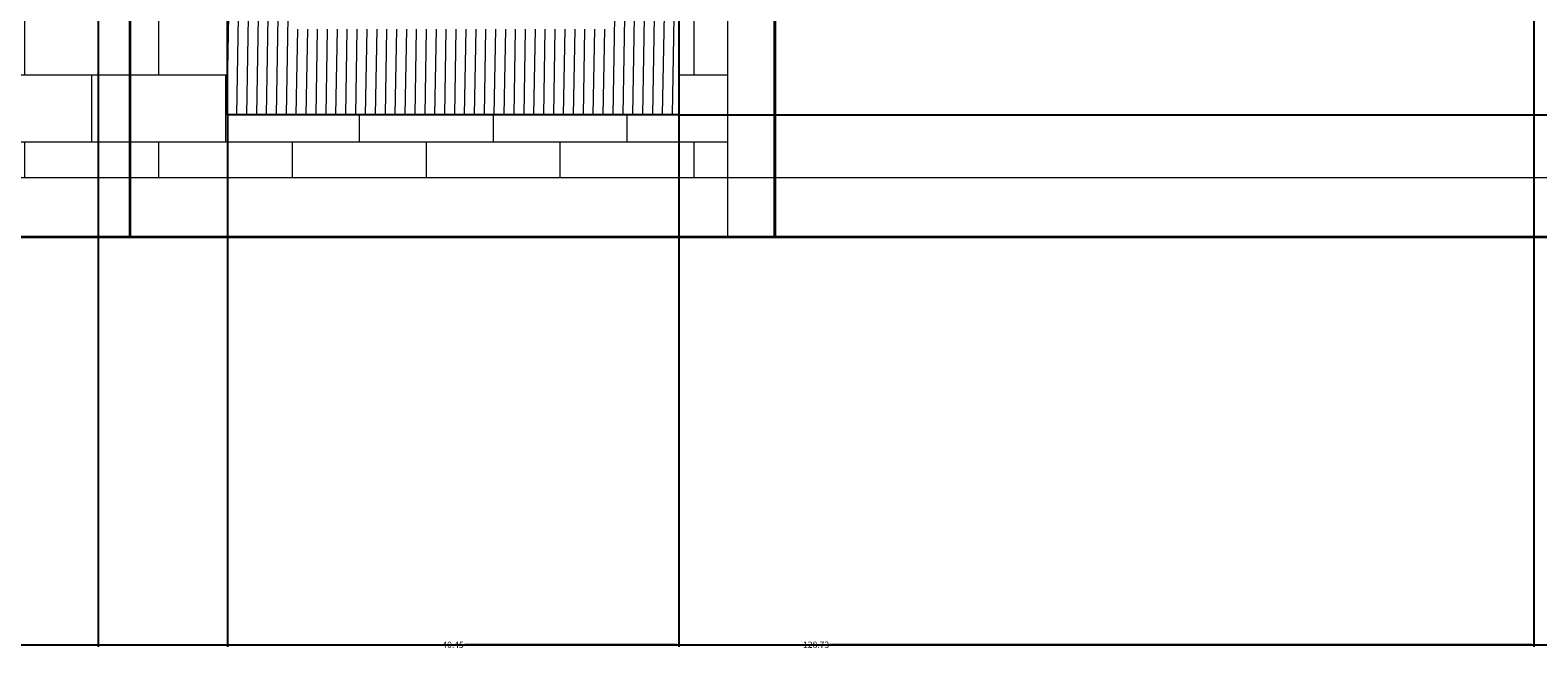
# Model space of a CAD drawing. Units: inches. Extents: x -26 to 776, y -22 to 650.
# Tile 14 of 62: x 222 to 358, y -22 to 34. Entities that reach past the tile are written whole.
import ezdxf

# ---------------------------------------------------------------- set-up
doc = ezdxf.new("R2010")
doc.units = ezdxf.units.IN
doc.header["$MEASUREMENT"] = 0
for name, color, linetype, lineweight in [('A-ANNO-DIMS', 2, 'Continuous', 18), ('A-DETL-PATT', 8, 'Continuous', 13), ('A-DOOR', 3, 'Continuous', 25), ('A-WALL', 7, 'Continuous', 35), ('A-WALL-PATT', 8, 'Continuous', 13), ('A-WALL-TRIM', 7, 'Continuous', 18), ('C-TOPO', 7, 'Continuous', 35)]:
    doc.layers.add(name, color=color, linetype=linetype, lineweight=lineweight)
doc.styles.get("Standard").update_dxf_attribs({"font": 'arial.ttf'})
doc.dimstyles.get("Standard").update_dxf_attribs({"dimtxt": 0.5625, "dimasz": 0.18, "dimexe": 0.18, "dimexo": 0.0625, "dimgap": 0.09, "dimtad": 0, "dimtih": 1, "dimtoh": 1, "dimdec": 4, "dimzin": 0, "dimdsep": 46, "dimlunit": 4, "dimtxsty": 'Standard', "dimcen": 0.09, "dimadec": 0, "dimazin": 0, "dimtfac": 1, "dimtdec": 4, "dimtofl": 0, "dimtmove": 0, "dimatfit": 3, "dimfxl": 1, "dimtolj": 1, "dimtzin": 0, "dimarcsym": 0})

# ---------------------------------------------------------------- blocks, each defined once
blk = doc.blocks.new('*D13')
at = {"layer": 'A-ANNO-DIMS', "color": 0, "lineweight": -2, "transparency": 16777216}
for p, q in [((738.75, 50.79), (738.75, -21.31)), ((11.11, 15.42), (11.11, -21.31)), ((11.29, -21.13), (373.89, -21.13)), ((738.57, -21.13), (375.97, -21.13))]:
    blk.add_line(p, q, dxfattribs=at)
at = {"layer": 'A-ANNO-DIMS', "color": 0, "transparency": 16777216}
for points in [[(11.29, -21.1), (11.29, -21.16), (11.11, -21.13)], [(738.57, -21.1), (738.57, -21.16), (738.75, -21.13)]]:
    blk.add_solid(points, dxfattribs=at)
at = {"layer": 'Defpoints', "color": 0, "transparency": 16777216}
for p in [(738.75, 50.85), (11.11, 15.48), (738.75, -21.13)]:
    blk.add_point(p, dxfattribs=at)
at = {"layer": 'A-ANNO-DIMS', "color": 0, "transparency": 16777216, "insert": (374.93, -21.13), "char_height": 0.562, "attachment_point": 5}
blk.add_mtext('\\A1;727.6', dxfattribs=at)
blk = doc.blocks.new('*D29')
at = {"layer": 'A-ANNO-DIMS', "color": 0, "lineweight": -2, "transparency": 16777216}
for p, q in [((240.17, 26.36), (240.17, -21.31)), ((280.62, 26.36), (280.62, -21.31)), ((240.35, -21.13), (259.34, -21.13)), ((280.44, -21.13), (261.44, -21.13))]:
    blk.add_line(p, q, dxfattribs=at)
at = {"layer": 'A-ANNO-DIMS', "color": 0, "transparency": 16777216}
for points in [[(240.35, -21.1), (240.35, -21.16), (240.17, -21.13)], [(280.44, -21.1), (280.44, -21.16), (280.62, -21.13)]]:
    blk.add_solid(points, dxfattribs=at)
at = {"layer": 'Defpoints', "color": 0, "transparency": 16777216}
for p in [(240.17, 26.42), (280.62, 26.42), (280.62, -21.13)]:
    blk.add_point(p, dxfattribs=at)
at = {"layer": 'A-ANNO-DIMS', "color": 0, "transparency": 16777216, "insert": (260.39, -21.13), "char_height": 0.562, "attachment_point": 5}
blk.add_mtext('\\A1;40.45', dxfattribs=at)
blk = doc.blocks.new('*D30')
at = {"layer": 'A-ANNO-DIMS', "color": 0, "lineweight": -2, "transparency": 16777216}
for p, q in [((280.68, 144.84), (775.34, 144.84)), ((775.16, 144.66), (775.16, 86.01)), ((775.16, 26.6), (775.16, 85.25)), ((280.68, 26.42), (775.34, 26.42))]:
    blk.add_line(p, q, dxfattribs=at)
at = {"layer": 'A-ANNO-DIMS', "color": 0, "transparency": 16777216}
for points in [[(775.13, 144.66), (775.19, 144.66), (775.16, 144.84)], [(775.13, 26.6), (775.19, 26.6), (775.16, 26.42)]]:
    blk.add_solid(points, dxfattribs=at)
at = {"layer": 'Defpoints', "color": 0, "transparency": 16777216}
for p in [(280.62, 144.84), (775.16, 144.84), (280.62, 26.42)]:
    blk.add_point(p, dxfattribs=at)
at = {"layer": 'A-ANNO-DIMS', "color": 0, "transparency": 16777216, "insert": (775.16, 85.63), "char_height": 0.562, "attachment_point": 5}
blk.add_mtext('\\A1;118.41', dxfattribs=at)
blk = doc.blocks.new('*D34')
at = {"layer": 'A-ANNO-DIMS', "color": 0, "lineweight": -2, "transparency": 16777216}
for p, q in [((228.57, 528.3), (228.57, -21.31)), ((357.3, 528.36), (357.3, -21.31)), ((228.75, -21.13), (291.71, -21.13)), ((357.12, -21.13), (294.17, -21.13))]:
    blk.add_line(p, q, dxfattribs=at)
at = {"layer": 'A-ANNO-DIMS', "color": 0, "transparency": 16777216}
for points in [[(228.75, -21.1), (228.75, -21.16), (228.57, -21.13)], [(357.12, -21.1), (357.12, -21.16), (357.3, -21.13)]]:
    blk.add_solid(points, dxfattribs=at)
at = {"layer": 'Defpoints', "color": 0, "transparency": 16777216}
for p in [(228.57, 528.36), (357.3, 528.42), (357.3, -21.13)]:
    blk.add_point(p, dxfattribs=at)
at = {"layer": 'A-ANNO-DIMS', "color": 0, "transparency": 16777216, "insert": (292.94, -21.13), "char_height": 0.562, "attachment_point": 5}
blk.add_mtext('\\A1;128.73', dxfattribs=at)
blk = doc.blocks.new('*D37')
at = {"layer": 'A-ANNO-DIMS', "color": 0, "lineweight": -2, "transparency": 16777216}
for p, q in [((231.36, 159.48), (-25.48, 159.48)), ((-25.3, 159.3), (-25.3, 87.85)), ((-25.3, 15.66), (-25.3, 87.11)), ((217.89, 15.48), (-25.48, 15.48))]:
    blk.add_line(p, q, dxfattribs=at)
at = {"layer": 'A-ANNO-DIMS', "color": 0, "transparency": 16777216}
for points in [[(-25.33, 159.3), (-25.27, 159.3), (-25.3, 159.48)], [(-25.33, 15.66), (-25.27, 15.66), (-25.3, 15.48)]]:
    blk.add_solid(points, dxfattribs=at)
at = {"layer": 'Defpoints', "color": 0, "transparency": 16777216}
for p in [(-25.3, 159.48), (231.42, 159.48), (217.95, 15.48)]:
    blk.add_point(p, dxfattribs=at)
at = {"layer": 'A-ANNO-DIMS', "color": 0, "transparency": 16777216, "insert": (-25.3, 87.48), "char_height": 0.562, "attachment_point": 5}
blk.add_mtext('\\A1;144', dxfattribs=at)
blk = doc.blocks.new('*D38')
at = {"layer": 'A-ANNO-DIMS', "color": 0, "lineweight": -2, "transparency": 16777216}
for p, q in [((280.68, 26.42), (775.34, 26.42)), ((775.16, 26.24), (775.16, 21.33)), ((775.16, 15.66), (775.16, 20.58)), ((289.3, 15.48), (775.34, 15.48))]:
    blk.add_line(p, q, dxfattribs=at)
at = {"layer": 'A-ANNO-DIMS', "color": 0, "transparency": 16777216}
for points in [[(775.13, 26.24), (775.19, 26.24), (775.16, 26.42)], [(775.13, 15.66), (775.19, 15.66), (775.16, 15.48)]]:
    blk.add_solid(points, dxfattribs=at)
at = {"layer": 'Defpoints', "color": 0, "transparency": 16777216}
for p in [(280.62, 26.42), (775.16, 26.42), (289.24, 15.48)]:
    blk.add_point(p, dxfattribs=at)
at = {"layer": 'A-ANNO-DIMS', "color": 0, "transparency": 16777216, "insert": (775.16, 20.95), "char_height": 0.562, "attachment_point": 5}
blk.add_mtext('\\A1;10.942', dxfattribs=at)
blk = doc.blocks.new('*D39')
at = {"layer": 'A-ANNO-DIMS', "color": 0, "lineweight": -2, "transparency": 16777216}
for p, q in [((289.24, 15.54), (289.24, 649.86)), ((289.42, 649.68), (356.48, 649.68)), ((425.56, 649.68), (358.51, 649.68)), ((425.74, 15.54), (425.74, 649.86))]:
    blk.add_line(p, q, dxfattribs=at)
at = {"layer": 'A-ANNO-DIMS', "color": 0, "transparency": 16777216}
for points in [[(289.42, 649.71), (289.42, 649.65), (289.24, 649.68)], [(425.56, 649.71), (425.56, 649.65), (425.74, 649.68)]]:
    blk.add_solid(points, dxfattribs=at)
at = {"layer": 'Defpoints', "color": 0, "transparency": 16777216}
for p in [(425.74, 649.68), (289.24, 15.48), (425.74, 15.48)]:
    blk.add_point(p, dxfattribs=at)
at = {"layer": 'A-ANNO-DIMS', "color": 0, "transparency": 16777216, "insert": (357.49, 649.68), "char_height": 0.562, "attachment_point": 5}
blk.add_mtext('\\A1;136.5', dxfattribs=at)
blk = doc.blocks.new('*D44')
at = {"layer": 'A-ANNO-DIMS', "color": 0, "lineweight": -2, "transparency": 16777216}
for p, q in [((231.42, 15.54), (231.42, 649.86)), ((231.6, 649.68), (234.98, 649.68)), ((239.99, 649.68), (236.61, 649.68)), ((240.17, 26.49), (240.17, 649.86))]:
    blk.add_line(p, q, dxfattribs=at)
at = {"layer": 'A-ANNO-DIMS', "color": 0, "transparency": 16777216}
for points in [[(231.6, 649.71), (231.6, 649.65), (231.42, 649.68)], [(239.99, 649.71), (239.99, 649.65), (240.17, 649.68)]]:
    blk.add_solid(points, dxfattribs=at)
at = {"layer": 'Defpoints', "color": 0, "transparency": 16777216}
for p in [(240.17, 649.68), (240.17, 26.42), (231.42, 15.48)]:
    blk.add_point(p, dxfattribs=at)
at = {"layer": 'A-ANNO-DIMS', "color": 0, "transparency": 16777216, "insert": (235.8, 649.68), "char_height": 0.562, "attachment_point": 5}
blk.add_mtext('\\A1;8.74', dxfattribs=at)

msp = doc.modelspace()

# ---------------------------------------------------------------- hatches: boundary and pattern name
at = {"layer": 'A-DETL-PATT'}
h = msp.add_hatch(dxfattribs=at)
h.set_pattern_fill('ANSI31', color=256, scale=7.1, angle=44)
h.paths.add_polyline_path([(231.4249, 197.3298), (216.1056, 197.3298), (216.1056, 159.4824), (231.4249, 159.4824)])
h.paths.add_polyline_path([(236.4647, 197.3298), (231.4249, 197.3298), (231.4249, 159.4824), (276.1134, 159.4824), (276.1134, 171.4173), (236.4647, 171.4173)])
h.paths.add_polyline_path([(259.7413, 197.3298), (236.4647, 197.3298), (236.4647, 171.4173), (259.7413, 171.4173)], flags=17)
h.paths.add_polyline_path([(276.1134, 197.3298), (261.7413, 197.3298), (261.7413, 171.4173), (276.1134, 171.4173)], flags=17)
h.paths.add_polyline_path([(217.9529, 147.0781), (22.8891, 147.0781), (22.8891, 138.3844), (217.9529, 138.3844)])
h.paths.add_polyline_path([(285.0179, 152.3087), (285.0179, 159.4824), (231.4249, 159.4824), (240.1654, 144.8359), (280.6173, 144.8359)])
h.paths.add_polyline_path([(280.6173, 144.8359), (240.1654, 144.8359), (240.1654, 26.4239), (280.6173, 26.4239)])
h.paths.add_polyline_path([(274.6644, 134.8811), (274.6644, 34.0885), (245.7207, 34.0885), (245.7207, 134.8811)], flags=16)
h.paths.add_polyline_path([(285.0179, 303.3046), (236.4647, 303.3046), (236.4647, 294.4171), (285.0179, 294.4171)])
h.paths.add_polyline_path([(285.0179, 446.0063), (236.4647, 446.0063), (236.4647, 437.1188), (285.0179, 437.1188)])
at = {"layer": 'A-WALL-PATT'}
h = msp.add_hatch(dxfattribs=at)
h.set_pattern_fill('AR-B816', color=256, scale=4.5)
h.paths.add_polyline_path([(425.7434, 448.2114), (289.2424, 496.9554), (289.2424, 458.1203), (289.2424, 291.1798), (289.2424, 20.7937), (425.7434, 20.7937), (425.7434, 283.2492)])
h = msp.add_hatch(dxfattribs=at)
h.set_pattern_fill('AR-B816', color=256, scale=0.75)
h.paths.add_polyline_path([(82.134, 209.6413), (11.1074, 209.6413), (11.1074, 159.4824), (82.134, 159.4824)])
h.paths.add_polyline_path([(231.4249, 209.6413), (209.091, 209.6413), (209.091, 159.4824), (214.1056, 159.4824), (214.1056, 199.3298), (231.4249, 199.3298)])
h.paths.add_polyline_path([(231.4249, 159.4824), (11.1074, 159.4824), (11.1074, 22.5014), (22.8891, 22.5014), (22.8891, 147.0781), (217.9529, 147.0781), (217.9529, 20.7937), (231.4249, 20.7937)])
h.paths.add_polyline_path([(285.0179, 152.3087), (280.6173, 144.8359), (280.6173, 26.4239), (240.1654, 26.4239), (240.1654, 144.8359), (231.4249, 159.4824), (231.4249, 20.7937), (285.0179, 20.7937)])

# ---------------------------------------------------------------- linework, layer by layer
at = {"layer": 'A-DOOR'}
msp.add_lwpolyline([(240.1654, 144.8359), (280.6173, 144.8359), (280.6173, 26.4239), (240.1654, 26.4239)], close=True, dxfattribs=at)
at = {"layer": 'A-WALL'}
for p, q in [((289.2424, 291.1798), (289.2424, 15.4824)), ((231.4249, 159.4824), (231.4249, 15.4824)), ((289.2424, 15.4824), (289.2424, 159.4824))]:
    msp.add_line(p, q, dxfattribs=at)
at = {"layer": 'A-WALL-TRIM'}
for p, q in [((285.0179, 15.4824), (285.0179, 249.6598)), ((217.9529, 20.7937), (425.7434, 20.7937))]:
    msp.add_line(p, q, dxfattribs=at)
at = {"layer": 'C-TOPO'}
for p, q in [((214.0443, 15.4824), (289.2424, 15.4824)), ((289.2424, 15.4824), (425.7434, 15.4824))]:
    msp.add_line(p, q, dxfattribs=at)

# ---------------------------------------------------------------- dimensions: what is measured, and where the dimension line sits
at = {"layer": 'A-ANNO-DIMS'}
for base, p1, p2, override, picture, middle in [((240.1654, 649.6763), (231.4249, 15.4824), (240.1654, 26.4239), {"dimdec": 2, "dimlfac": 1, "dimrnd": 0, "dimzin": 0, "dimdsep": 46, "dimlunit": 2}, '*D44', (235.7952, 649.6763)), ((425.7434, 649.6763), (289.2424, 15.4824), (425.7434, 15.4824), {"dimdec": 1, "dimlfac": 1, "dimrnd": 0, "dimzin": 0, "dimdsep": 46, "dimlunit": 2}, '*D39', (357.4929, 649.6763)), ((357.3034, -21.1349), (228.5733, 528.3585), (357.3034, 528.4233), {"dimdec": 2, "dimlfac": 1, "dimrnd": 0, "dimzin": 0, "dimdsep": 46, "dimlunit": 2}, '*D34', (292.9384, -21.1349)), ((738.7503, -21.1349), (11.1074, 15.4824), (738.7503, 50.8482), {"dimdec": 1, "dimlfac": 1, "dimrnd": 0, "dimzin": 0, "dimdsep": 46, "dimlunit": 2}, '*D13', (374.9289, -21.1349)), ((280.6173, -21.1349), (240.1654, 26.4239), (280.6173, 26.4239), {"dimdec": 2, "dimlfac": 1, "dimrnd": 0, "dimzin": 0, "dimdsep": 46, "dimlunit": 2}, '*D29', (260.3914, -21.1349))]:
    dim = msp.add_linear_dim(base=base, p1=p1, p2=p2, dimstyle='Standard', override=override, dxfattribs=at)
    dim.commit()
    dim.dimension.update_dxf_attribs({"geometry": picture, "text_midpoint": middle})
for base, p1, p2, override, picture, middle in [((-25.2976, 159.4824), (217.9529, 15.4824), (231.4249, 159.4824), {"dimdec": 0, "dimlfac": 1, "dimrnd": 0, "dimzin": 0, "dimdsep": 46, "dimlunit": 2}, '*D37', (-25.2976, 87.4824)), ((775.1553, 144.8359), (280.6173, 26.4239), (280.6173, 144.8359), {"dimdec": 2, "dimlfac": 1, "dimrnd": 0, "dimzin": 0, "dimdsep": 46, "dimlunit": 2}, '*D30', (775.1553, 85.6299)), ((775.15535, 26.4239), (289.24236, 15.48237), (280.61732, 26.4239), {"dimdec": 3, "dimlfac": 1, "dimrnd": 0, "dimzin": 0, "dimdsep": 46, "dimlunit": 2}, '*D38', (775.15535, 20.95313))]:
    dim = msp.add_linear_dim(base=base, p1=p1, p2=p2, angle=90, dimstyle='Standard', override=override, dxfattribs=at)
    dim.commit()
    dim.dimension.update_dxf_attribs({"geometry": picture, "text_midpoint": middle})

doc.saveas('drawing.dxf')
